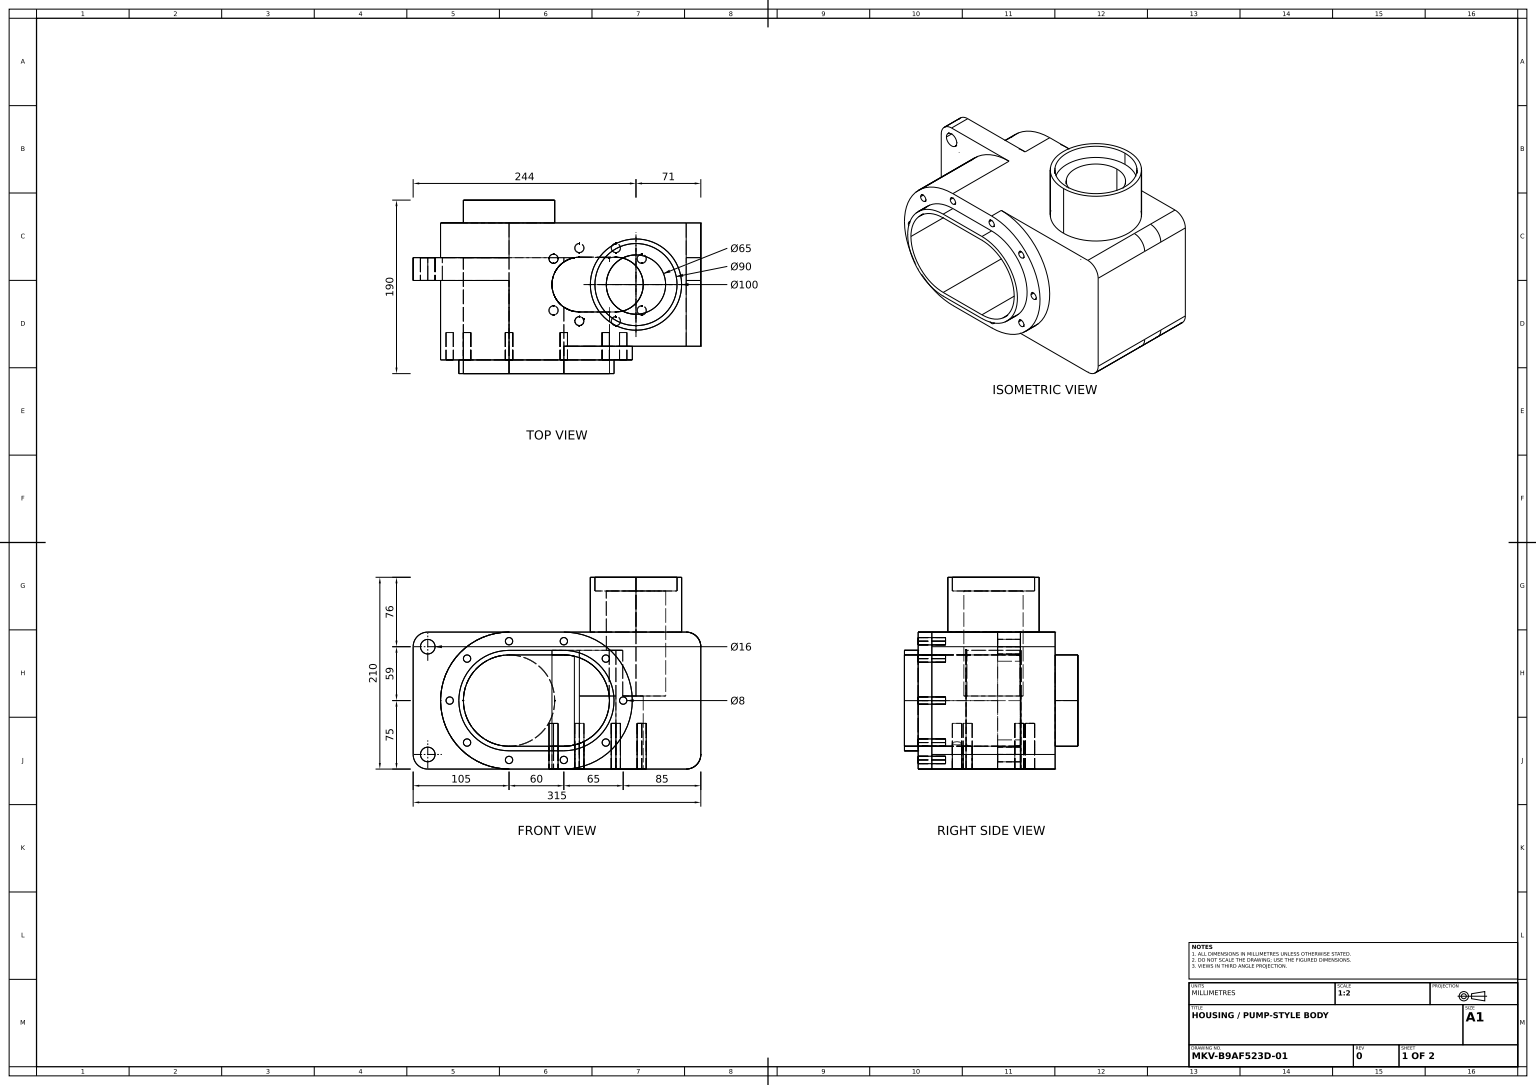
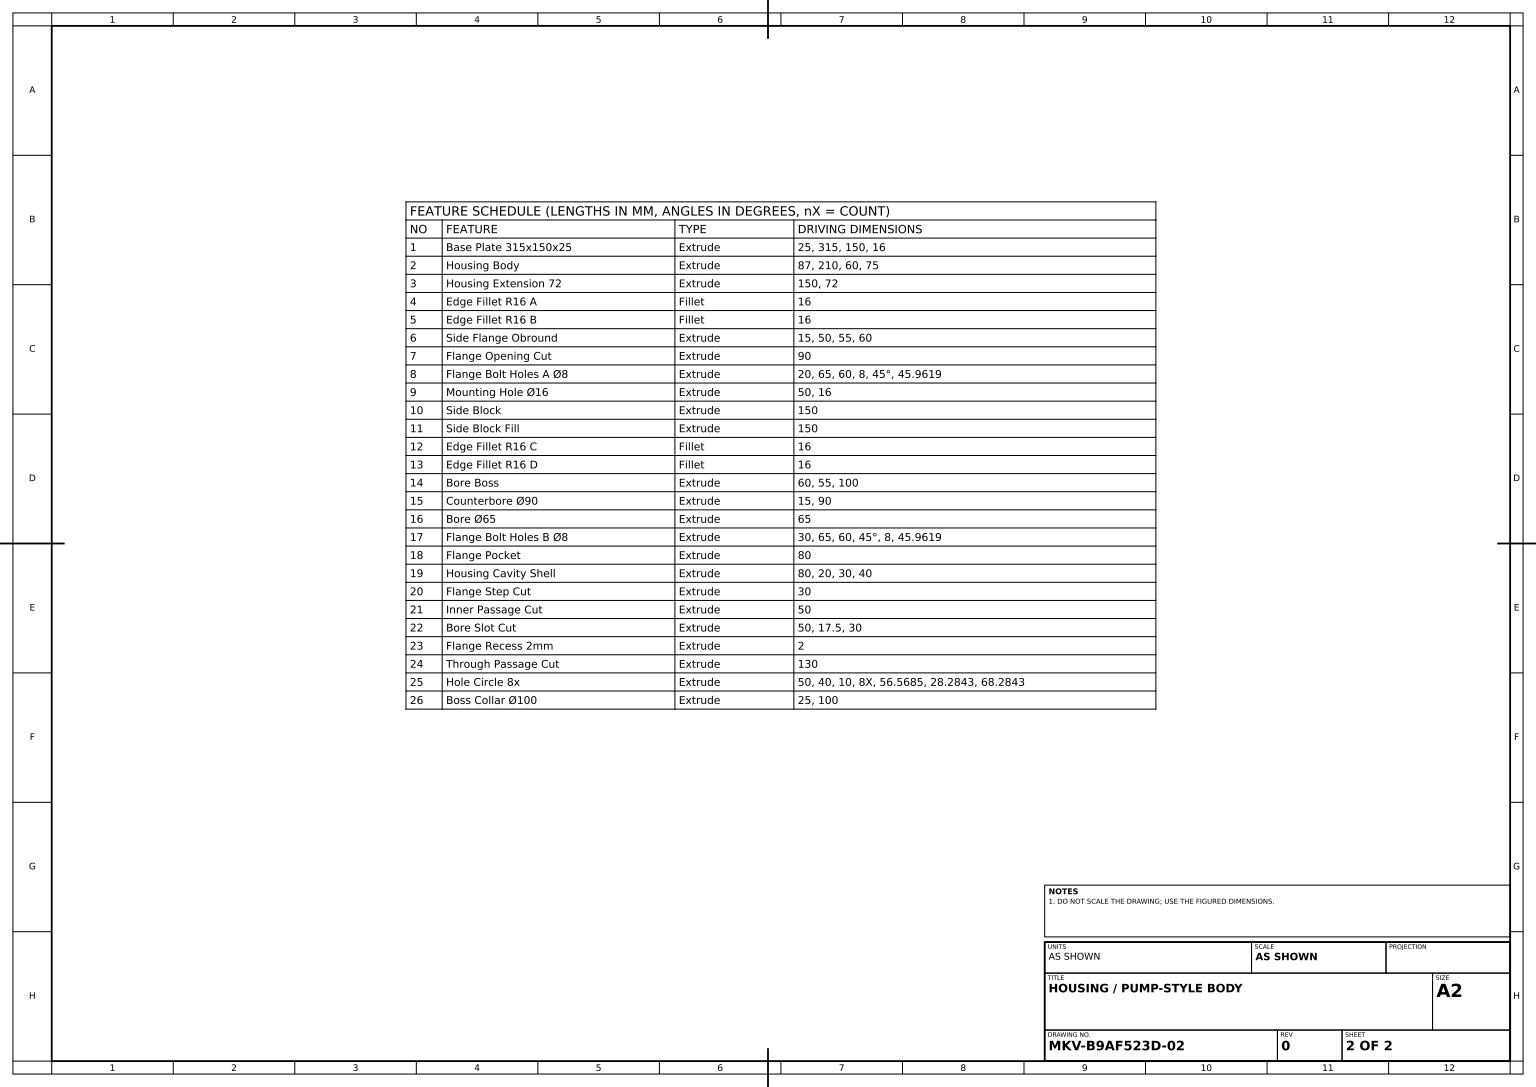
SolidWorks part; units mm, degrees
material "Plain Carbon Steel"
ref_plane "Front Plane" through (0, 0, 0) normal (0, 0, 1) x (1, 0, 0)
ref_plane "Top Plane" through (0, 0, 0) normal (0, 1, 0) x (1, 0, 0)
ref_plane "Right Plane" through (0, 0, 0) normal (1, 0, 0) x (0, 0, -1)
sketch "Base Plate Sketch" plane through (0, 0, 0) normal (0, 0, 1) x (1, 0, 0)
  line L0 (16, 0) -> (299, 0)
  line L1 (315, 16) -> (315, 134)
  line L2 (299, 150) -> (16, 150)
  line L3 (0, 134) -> (0, 16)
  arc A0 (16, 0) -> (0, 16) centre (16, 16) cw
  arc A1 (299, 0) -> (315, 16) centre (299, 16) ccw
  arc A2 (315, 134) -> (299, 150) centre (299, 134) ccw
  arc A3 (16, 150) -> (0, 134) centre (16, 134) ccw
  point P7 (0, 0)
  point P10 (315, 0)
  point P13 (315, 150)
  dimension "D3" = 16
  dimension "D1" = 315
  dimension "D2" = 150
extrude "Base Plate 315x150x25" add sketch "Base Plate Sketch" along normal blind 25
sketch "Housing Body Sketch" plane through (0, 0, 25) normal (0, 0, 1) x (1, 0, 0)
  line L0 (315, 75) -> (105, 75)
  line L1 (315, 16) -> (315, 134) construction
  line L2 (105, 150) -> (165, 150)
  line L3 (299, 150) -> (16, 150) construction
  line L5 (105, 0) -> (165, 0)
  arc A1 (165, 0) -> (165, 150) centre (165, 75) ccw
  arc A2 (105, 150) -> (105, 0) centre (105, 75) ccw
  dimension "D2" = 75
  dimension "D4" = 75
  dimension "D1" = 210
  dimension "D3" = 60
extrude "Housing Body" add sketch "Housing Body Sketch" along normal blind 87
sketch "Housing Extension Sketch" plane through (0, 0, 0) normal (0, -1, 0) x (1, 0, 0)
  line L0 (165, 25) -> (315, 25)
  line L1 (315, 25) -> (315, 97)
  line L2 (315, 97) -> (165, 97)
  line L3 (165, 112) -> (165, 25) construction
  line L4 (165, 97) -> (165, 25)
  dimension "D1" = 72
extrude "Housing Extension 72" add sketch "Housing Extension Sketch" against normal blind 150
fillet "Edge Fillet R16 A" radius 16 1 edges at (315, 0, 61)
fillet "Edge Fillet R16 B" radius 16 1 edges at (315, 150, 61)
sketch "Side Flange Sketch" plane through (0, 0, 112) normal (0, 0, 1) x (1, 0, 0)
  line L0 (105, 130) -> (165, 130)
  line L1 (105, 125) -> (165, 125)
  line L2 (105, 20) -> (165, 20)
  line L3 (105, 25) -> (165, 25)
  arc A0 (105, 125) -> (105, 25) centre (105, 75) ccw
  arc A1 (165, 25) -> (165, 125) centre (165, 75) ccw
  arc A2 (105, 130) -> (105, 20) centre (105, 75) ccw
  arc A3 (165, 20) -> (165, 130) centre (165, 75) ccw
  dimension "D1" = 50
  dimension "D2" = 50
  dimension "D3" = 55
  dimension "D4" = 55
  dimension "D5" = 60
  dimension "D6" = 60
  dimension "D7" = 60
  dimension "D8" = 60
extrude "Side Flange Obround" add sketch "Side Flange Sketch" along normal blind 15
sketch "Flange Opening Sketch" plane through (0, 0, 112) normal (0, 0, 1) x (1, 0, 0)
  line L0 (105, 125) -> (165, 125)
  line L1 (105, 25) -> (165, 25)
  arc A0 (105, 125) -> (105, 25) centre (105, 75) ccw
  arc A1 (165, 25) -> (165, 125) centre (165, 75) ccw
extrude "Flange Opening Cut" cut sketch "Flange Opening Sketch" against normal blind 90
sketch "Flange Bolt Holes A Sketch" plane through (0, 0, 112) normal (0, 0, 1) x (1, 0, 0)
  line L0 (105, 140) -> (165, 140)
  line L1 (105, 10) -> (165, 10)
  line L2 (40, 75) -> (230, 75)
  line L4 (165, 75) -> (210.9619, 120.9619)
  line L5 (165, 75) -> (210.9619, 29.0381)
  line L6 (105, 75) -> (59.0381, 120.9619)
  line L7 (105, 75) -> (59.0381, 29.0381)
  arc A0 (105, 140) -> (105, 10) centre (105, 75) ccw
  arc A1 (165, 10) -> (165, 140) centre (165, 75) ccw
  circle A2 centre (40, 75) radius 4
  circle A3 centre (230, 75) radius 4
  circle A4 centre (105, 140) radius 4
  circle A5 centre (165, 140) radius 4
  circle A6 centre (105, 10) radius 4
  circle A7 centre (165, 10) radius 4
  circle A8 centre (210.9619, 120.9619) radius 4
  circle A9 centre (59.0381, 120.9619) radius 4
  circle A10 centre (59.0381, 29.0381) radius 4
  circle A11 centre (210.9619, 29.0381) radius 4
  dimension "D1" = 65
  dimension "D2" = 65
  dimension "D5" = 8
  dimension "D6" = 8
  dimension "D7" = 8
  dimension "D8" = 8
  dimension "D9" = 8
  dimension "D10" = 8
  dimension "D15" = 8
  dimension "D16" = 8
  dimension "D17" = 8
  dimension "D18" = 8
  dimension "D3" = 60
  dimension "D4" = 60
  dimension "D11" = 45
  dimension "D12" = 45
  dimension "D13" = 45
  dimension "D14" = 45
  dimension "D19" = 45.9619
  dimension "D20" = 65
extrude "Flange Bolt Holes A Ø8" cut sketch "Flange Bolt Holes A Sketch" against normal blind 20 contours A0 A2 | A0 A2 L2 | L2 A2 A0 | A0 A10 | A0 A10 L7 | L7 A10 A0 | A0 A6 L1 | L1 A6 A0 | L1 A7 A1 | A1 A7 L1 | A1 A11 | L5 A11 A1 | A1 A11 L5 | A1 A3 | A1 A3 L2 | L2 A3 A1 | L4 A8 A1 | A1 A8 | A1 A8 L4 | L0 A5 A1 | A1 A5 L0 | A0 A4 L0 | L0 A4 A0 | L6 A9 A0 | A0 A9 L6 | A0 A9
sketch "Mounting Hole Sketch" plane through (0, 0, 25) normal (0, 0, 1) x (1, 0, 0)
  circle A0 centre (16, 134) radius 8
  circle A1 centre (16, 16) radius 8
  dimension "D1" = 16
  dimension "D2" = 16
extrude "Mounting Hole Ø16" cut sketch "Mounting Hole Sketch" against normal blind 50
sketch "Side Block Sketch" plane through (0, 0, 112) normal (0, 0, 1) x (1, 0, 0)
  line L0 (105, 150) -> (165, 150)
  line L1 (105, 0) -> (165, 0)
  arc A0 (105, 150) -> (105, 0) centre (105, 75) ccw
  arc A1 (165, 0) -> (165, 150) centre (165, 75) ccw
extrude "Side Block" add sketch "Side Block Sketch" against normal blind 150
sketch "Side Block Fill Sketch" plane through (0, 150, 0) normal (0, 1, 0) x (1, 0, 0)
  line L0 (165, 38) -> (315, 38)
  line L1 (315, 38) -> (315, 0)
  line L2 (315, 0) -> (165, 0)
  line L3 (165, 0) -> (165, 38)
extrude "Side Block Fill" add sketch "Side Block Fill Sketch" against normal blind 150
fillet "Edge Fillet R16 C" radius 16 1 edges at (315, 150, -19)
fillet "Edge Fillet R16 D" radius 16 1 edges at (315, 0, -19)
sketch "Bore Boss Sketch" plane through (0, 150, 0) normal (0, 1, 0) x (1, 0, 0)
  line L0 (299, 38) -> (299, -97)
  line L1 (299, -29.5) -> (244, -29.5)
  circle A0 centre (244, -29.5) radius 50
  dimension "D2" = 100
  dimension "D1" = 55
extrude "Bore Boss" add sketch "Bore Boss Sketch" along normal blind 60
sketch "Counterbore Sketch" plane through (0, 210, 0) normal (0, 1, 0) x (1, 0, 0)
  circle A0 centre (244, -29.5) radius 45
  dimension "D1" = 90
extrude "Counterbore Ø90" cut sketch "Counterbore Sketch" against normal blind 15
sketch "Bore Sketch" plane through (0, 195, 0) normal (0, 1, 0) x (1, 0, 0)
  circle A0 centre (244, -29.5) radius 32.5
  dimension "D1" = 65
extrude "Bore Ø65" cut sketch "Bore Sketch" against normal blind 65
sketch "Flange Bolt Holes B Sketch" plane through (0, 0, 112) normal (0, 0, 1) x (1, 0, 0)
  line L0 (105, 140) -> (165, 140)
  line L1 (105, 10) -> (165, 10)
  line L2 (40, 75) -> (230, 75)
  line L4 (105, 75) -> (59.0381, 120.9619)
  line L5 (105, 75) -> (59.0381, 29.0381)
  line L6 (165, 75) -> (210.9619, 120.9619)
  line L7 (165, 75) -> (210.9619, 29.0381)
  arc A0 (105, 140) -> (105, 10) centre (105, 75) ccw
  arc A1 (165, 10) -> (165, 140) centre (165, 75) ccw
  circle A2 centre (40, 75) radius 4
  circle A3 centre (59.0381, 120.9619) radius 4
  circle A4 centre (59.0381, 29.0381) radius 4
  circle A5 centre (210.9619, 120.9619) radius 4
  circle A6 centre (230, 75) radius 4
  circle A7 centre (210.9619, 29.0381) radius 4
  circle A8 centre (105, 140) radius 4
  circle A9 centre (165, 140) radius 4
  circle A10 centre (105, 10) radius 4
  circle A11 centre (165, 10) radius 4
  dimension "D1" = 65
  dimension "D2" = 65
  dimension "D9" = 8
  dimension "D10" = 8
  dimension "D11" = 8
  dimension "D12" = 8
  dimension "D13" = 8
  dimension "D14" = 8
  dimension "D15" = 8
  dimension "D16" = 8
  dimension "D17" = 8
  dimension "D18" = 8
  dimension "D3" = 60
  dimension "D4" = 60
  dimension "D5" = 45
  dimension "D6" = 45
  dimension "D7" = 45
  dimension "D8" = 45
  dimension "D19" = 45.9619
  dimension "D20" = 65
extrude "Flange Bolt Holes B Ø8" cut sketch "Flange Bolt Holes B Sketch" against normal blind 30 contours A0 A2 | A0 A2 L2 | L2 A2 A0 | A0 A3 | L4 A3 A0 | A0 A3 L4 | L0 A8 A0 | A0 A8 L0 | A1 A9 L0 | L0 A9 A1 | A1 A5 | A1 A5 L6 | L6 A5 A1 | A1 A6 | A1 A6 L2 | L2 A6 A1 | A1 A7 | L7 A7 A1 | A1 A7 L7 | A1 A11 L1 | L1 A11 A1 | L1 A10 A0 | A0 A10 L1 | A0 A4 L5 | L5 A4 A0 | A0 A4
sketch "Flange Pocket Sketch" plane through (0, 0, 112) normal (0, 0, 1) x (1, 0, 0)
  line L0 (105, 125) -> (165, 125)
  line L1 (105, 25) -> (165, 25)
  arc A0 (105, 125) -> (105, 25) centre (105, 75) ccw
  arc A1 (165, 25) -> (165, 125) centre (165, 75) ccw
extrude "Flange Pocket" cut sketch "Flange Pocket Sketch" against normal blind 80
sketch "Housing Cavity Sketch" plane through (0, 0, 0) normal (0, -1, 0) x (1, 0, 0)
  line L0 (299, 97) -> (299, -38)
  line L1 (299, 29.5) -> (105, 29.5)
  line L2 (105, 112) -> (105, 25) construction
  line L3 (202, 29.5) -> (222, 29.5)
  line L4 (202, 29.5) -> (182, 29.5)
  line L5 (182, 59.5) -> (222, 59.5)
  line L6 (182, -0.5) -> (222, -0.5)
  arc A0 (182, 59.5) -> (182, -0.5) centre (182, 29.5) ccw
  arc A1 (222, -0.5) -> (222, 59.5) centre (222, 29.5) ccw
  dimension "D3" = 30
  dimension "D4" = 30
  dimension "D1" = 20
  dimension "D2" = 20
  dimension "D5" = 40
  dimension "D6" = 40
extrude "Housing Cavity Shell" cut sketch "Housing Cavity Sketch" against normal blind 80 contours L1 A1 L5 A0 | L6 A1 L1 A0
sketch "Flange Step Sketch" plane through (0, 0, 32) normal (0, 0, 1) x (1, 0, 0)
  line L0 (105, 125) -> (165, 125)
  line L1 (105, 25) -> (165, 25)
  arc A0 (105, 125) -> (105, 25) centre (105, 75) ccw
  arc A1 (165, 25) -> (165, 125) centre (165, 75) ccw
extrude "Flange Step Cut" cut sketch "Flange Step Sketch" against normal blind 30
sketch "Inner Passage Sketch" plane through (0, 80, 0) normal (0, -1, 0) x (1, 0, 0)
  line L0 (214.7494, 59.5) -> (214.7494, 2)
  line L1 (214.7494, 59.5) -> (222, 59.5)
  line L2 (214.7494, 2) -> (214.7494, 0.3894)
  arc A0 (214.7494, 0.3894) -> (222, 59.5) centre (222, 29.5) ccw
extrude "Inner Passage Cut" cut sketch "Inner Passage Sketch" against normal blind 50
sketch "Bore Slot Sketch" plane through (0, 130, 0) normal (0, 1, 0) x (1, 0, 0)
  arc A0 (229.4489, -58.5605) -> (229.4489, -0.4395) centre (244, -29.5) ccw
  arc A1 (229.4489, -58.5605) -> (229.4489, -0.4395) centre (222, -29.5) ccw
  circle A2 centre (244, -29.5) radius 50 construction
  dimension "D1" = 17.5
  dimension "D2" = 30
extrude "Bore Slot Cut" cut sketch "Bore Slot Sketch" against normal blind 50
sketch "Flange Recess Sketch" plane through (0, 0, 2) normal (0, 0, 1) x (1, 0, 0)
  line L0 (105, 125) -> (165, 125)
  line L1 (105, 25) -> (165, 25)
  arc A0 (105, 125) -> (105, 25) centre (105, 75) ccw
  arc A1 (165, 25) -> (165, 125) centre (165, 75) ccw
extrude "Flange Recess 2mm" cut sketch "Flange Recess Sketch" against normal blind 2
sketch "Through Passage Sketch" plane through (0, 0, 0) normal (0, -1, 0) x (1, 0, 0)
  line L0 (214.7494, 59.5) -> (214.7494, 0)
  line L1 (214.7494, 0) -> (182, -0.5)
  line L2 (182, 59.5) -> (214.7494, 59.5)
  arc A0 (182, 59.5) -> (182.9158, -0.486) centre (182, 29.5) ccw
  arc M2 (182, -0.5) -> (182, 59.5) centre (182, 29.5) cw
  line M3 (182, 59.5) -> (222, 59.5)
extrude "Through Passage Cut" cut sketch "Through Passage Sketch" against normal blind 130 contours L1 L0 M3 M2
sketch "Hole Circle 8x Sketch" plane through (0, 0, 0) normal (0, -1, 0) x (1, 0, 0)
  line L0 (182, 69.5) -> (222, 69.5)
  line L1 (182, -10.5) -> (222, -10.5)
  arc A0 (182, 69.5) -> (182, -10.5) centre (182, 29.5) ccw
  arc A1 (222, -10.5) -> (222, 69.5) centre (222, 29.5) ccw
  circle A2 centre (222, 69.5) radius 5
  circle A3 centre (250.2843, 57.7843) radius 5
  circle A5 centre (250.2843, 1.2157) radius 5
  circle A6 centre (222, -10.5) radius 5
  circle A10 centre (182, 69.5) radius 5
  circle A14 centre (182, -10.5) radius 5
  circle A15 centre (153.7157, 1.2157) radius 5
  circle A17 centre (153.7157, 57.7843) radius 5
  circle A18 centre (222, 29.5) radius 5 [skipped]
  circle A19 centre (182, 29.5) radius 5 [skipped]
  circle A20 centre (142, 29.5) radius 5 [skipped]
  circle A21 centre (193.7157, 1.2157) radius 5 [skipped]
  circle A22 centre (193.7157, 57.7843) radius 5 [skipped]
  circle A23 centre (210.2843, 57.7843) radius 5 [skipped]
  circle A24 centre (210.2843, 1.2157) radius 5 [skipped]
  circle A25 centre (262, 29.5) radius 5 [skipped]
  dimension "D1" = 40
  dimension "D2" = 40
  dimension "D5" = 10
  dimension "D7" = 10
  dimension "D3" = 40
  dimension "D4" = 40
  dimension "D9" = 56.5685
  dimension "D10" = 28.2843
  dimension "D11" = 56.5685
  dimension "D12" = 68.2843
  dimension "D6" = 8
  dimension "D8" = 8
extrude "Hole Circle 8x" cut sketch "Hole Circle 8x Sketch" against normal blind 50 contours A0 A15 | A0 A15 | A0 A14 L1 | L1 A14 A0 | L1 A6 A1 | A1 A6 L1 | A1 A5 | A1 A5 | A1 A3 | A1 A3 | L0 A2 A1 | A1 A2 L0 | A0 A10 L0 | L0 A10 A0 | A0 A17
sketch "Boss Collar Sketch" plane through (0, 0, -38) normal (0, 0, -1) x (-1, 0, 0)
  circle A0 centre (-105, 75) radius 50
  dimension "D1" = 100
extrude "Boss Collar Ø100" add sketch "Boss Collar Sketch" along normal blind 25
